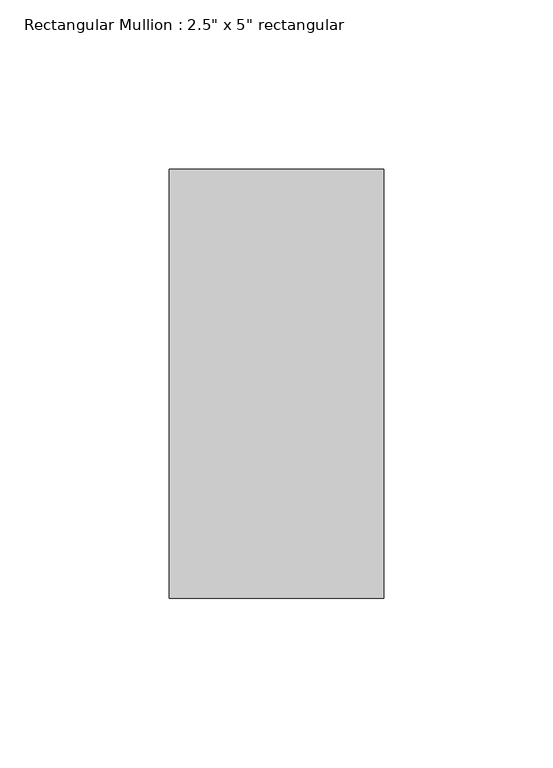
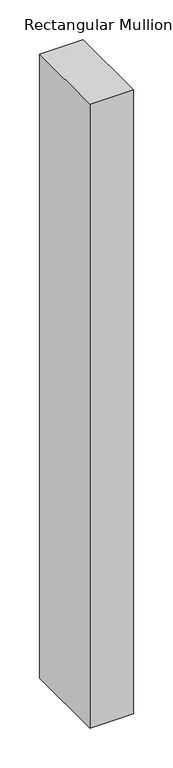
"""IFC4 building model written with IfcOpenShell, lengths in millimetres: member geometry."""

from ifc_helpers import new_model, si_unit, frame, origin, place, context, project, spatial, polyline, outline, extrude, source, transform, mapped, element, save


def member_fdbefc00(model_context):
    return source(origin(), model_context, "Body", "SweptSolid", [
        extrude(outline(polyline([(31.75, 63.5), (31.75, -63.5), (-31.75, -63.5), (-31.75, 63.5), (31.75, 63.5)])), frame((0.0, 0.0, -960.3935076), z_axis=(0.0, 0.0, 1.0), x_axis=(1.0, 0.0, 0.0)), (0.0, 0.0, 1.0), 960.3935076),
    ])


if __name__ == "__main__":
    model = new_model("IFC4")
    model_context = context("Model", 3, world=origin())
    ifc_project = project(units=[si_unit("LENGTHUNIT", "METRE", prefix="MILLI")], contexts=[model_context])
    site = spatial("IfcSite", under=ifc_project)
    building = spatial("IfcBuilding", under=site)
    placement = place(None, origin())
    member_shape = member_fdbefc00(model_context)
    element("IfcMember", 1, ObjectType="Rectangular Mullion : 2.5\" x 5\" rectangular", at=placement, inside=building, context=model_context, shape_type="MappedRepresentation", body=[
        mapped(member_shape, transform((0.0, 0.0, 0.0), x_axis=(1.0, 0.0, 0.0), y_axis=(0.0, 1.0, 0.0), z_axis=(0.0, 0.0, 1.0))),
    ])
    save(model, "model.ifc")

# Revit data of these elements
# Type "Rectangular Mullion : 2.5\" x 5\" rectangular"
#   built-in parameter 1007304 = 0.416667 (stored number, unit not read)
#   built-in parameter 1007301 = 0.104167 (stored number, unit not read)
#   built-in parameter 1007300 = 0.104167 (stored number, unit not read)
# Element 1 (IfcMember, "Rectangular Mullion : 2.5\" x 5\" rectangular")
#   Materials on its faces: "Aluminum"
# Materials
#   "Aluminum": class "Metal", colour RGB 247 247 247, transparency 0, Description = "Aluminum 6061", Cost = 0
